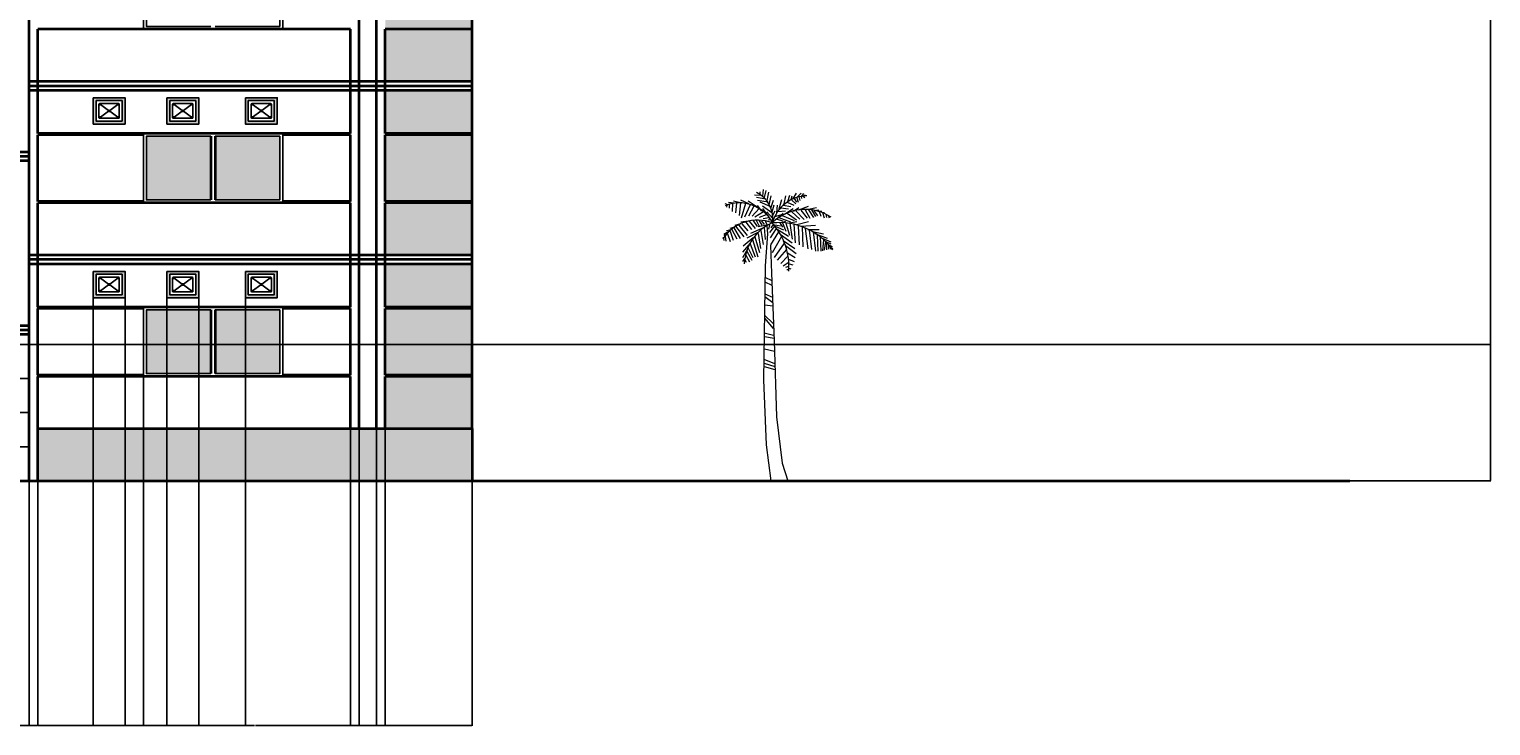
# Model space of a CAD drawing. Units: inches. Extents: x -742 to 1386, y -64 to 951.
# Tile 7 of 8: x 376 to 1386, y -64 to 418. Entities that reach past the tile are written whole.
import ezdxf

# ---------------------------------------------------------------- set-up
doc = ezdxf.new("R2010")
doc.units = ezdxf.units.IN
doc.header["$MEASUREMENT"] = 0
for name, color, linetype, lineweight in [('A-ANNO-DIMS', 2, 'Continuous', 18), ('A-DOOR', 31, 'Continuous', 25), ('A-ELEV', 7, 'Continuous', 35), ('A-ELEV-PATT', 252, 'Continuous', 13), ('A-GLAZ', 4, 'Continuous', 25), ('A-WALL-PATT', 8, 'Continuous', 13), ('tree', 3, 'Continuous', 18)]:
    doc.layers.add(name, color=color, linetype=linetype, lineweight=lineweight)
doc.styles.get("Standard").update_dxf_attribs({"font": 'arial.ttf'})
doc.dimstyles.get("Standard").update_dxf_attribs({"dimtxt": 0.18, "dimasz": 0.18, "dimexe": 0.18, "dimexo": 0.0625, "dimgap": 0.09, "dimtad": 0, "dimtih": 1, "dimtoh": 1, "dimdec": 4, "dimzin": 0, "dimdsep": 46, "dimtxsty": 'Standard', "dimcen": 0.09, "dimadec": 0, "dimazin": 0, "dimtfac": 1, "dimtdec": 4, "dimtofl": 0, "dimtmove": 0, "dimatfit": 3, "dimfxl": 1, "dimtolj": 1, "dimtzin": 0, "dimarcsym": 0})

# ---------------------------------------------------------------- blocks, each defined once
blk = doc.blocks.new('*U2')
for p, q in [((-25.283, 191.751), (-29.342, 192.246)), ((-20.064, 191.751), (-25.863, 193.238)), ((-21.031, 191.998), (-21.804, 183.325)), ((-15.232, 191.255), (-20.644, 193.981)), ((-9.433, 189.025), (-15.618, 193.238)), ((-6.727, 197.202), (-11.366, 197.45)), ((-3.441, 194.477), (-10.013, 195.716)), ((-1.894, 192.494), (-9.24, 193.733)), ((-7.5, 199.68), (-7.5, 197.946)), ((-0.541, 189.52), (-7.307, 192.494)), ((-5.567, 196.707), (-4.987, 201.167)), ((-4.407, 195.716), (-3.247, 200.672)), ((-2.474, 193.733), (-1.315, 199.433)), ((-1.121, 190.759), (0.232, 196.955)), ((0.038, 188.281), (1.778, 193.981)), ((5.837, 187.786), (7.577, 194.229)), ((9.317, 191.255), (10.283, 196.955)), ((11.25, 192.494), (15.889, 190.512)), ((11.829, 192.99), (13.182, 197.45)), ((13.956, 194.229), (14.729, 196.955)), ((14.536, 193.981), (17.242, 191.255)), ((15.116, 194.477), (17.822, 198.689)), ((16.082, 194.972), (17.822, 192.494)), ((18.015, 195.716), (20.914, 198.689)), ((18.015, 195.468), (18.981, 192.494)), ((19.368, 196.459), (19.948, 193.733)), ((20.914, 196.459), (21.301, 194.972)), ((21.301, 196.459), (22.847, 198.441)), ((22.074, 196.707), (23.427, 195.716)), ((23.234, 196.707), (23.62, 197.698)), ((-29.729, 190.759), (-31.469, 191.255)), ((-30.309, 190.512), (-30.695, 189.025)), ((-28.763, 190.759), (-28.763, 188.281)), ((-26.443, 191.503), (-26.636, 186.051)), ((-23.737, 191.751), (-24.51, 185.06)), ((-17.551, 191.503), (-20.451, 181.343)), ((-14.265, 190.759), (-18.131, 182.086)), ((-11.753, 189.768), (-15.425, 182.83)), ((-8.08, 188.034), (-12.912, 182.83)), ((-4.987, 185.803), (-10.979, 182.086)), ((-6.147, 186.299), (-9.24, 190.264)), ((-3.247, 183.821), (-8.08, 181.838)), ((-5.76, 190.016), (0.618, 185.308)), ((-5.76, 188.034), (-1.508, 182.582)), ((-2.668, 185.803), (1.198, 181.343)), ((1.005, 185.803), (2.358, 190.759)), ((1.005, 182.582), (2.938, 186.547)), ((2.938, 182.582), (6.61, 183.821)), ((4.098, 185.06), (4.678, 190.512)), ((4.871, 186.051), (10.09, 186.547)), ((4.871, 181.591), (8.544, 184.812)), ((5.644, 181.838), (13.569, 178.865)), ((6.997, 188.529), (12.216, 187.786)), ((7.77, 183.325), (16.082, 179.856)), ((8.544, 190.512), (13.763, 189.52)), ((9.51, 184.317), (15.502, 188.034)), ((11.25, 184.812), (17.628, 180.352)), ((14.536, 185.803), (19.948, 180.847)), ((15.695, 186.299), (19.368, 188.777)), ((17.242, 186.547), (23.041, 180.599)), ((19.368, 187.29), (26.133, 189.768)), ((20.721, 187.042), (25.167, 181.343)), ((23.814, 187.29), (26.907, 181.343)), ((24.78, 187.538), (31.546, 188.777)), ((26.133, 187.29), (29.419, 181.838)), ((28.066, 187.29), (30.966, 182.582)), ((29.806, 186.795), (32.319, 183.078)), ((29.999, 186.795), (33.092, 187.29)), ((32.512, 186.299), (35.218, 186.299)), ((33.479, 186.051), (34.445, 182.83)), ((35.605, 185.556), (37.151, 185.308)), ((35.798, 185.308), (36.958, 181.591)), ((38.118, 184.317), (38.504, 181.838)), ((39.857, 182.83), (40.244, 181.591)), ((-28.956, 172.174), (-32.435, 170.192)), ((-27.409, 173.413), (-30.695, 172.67)), ((-25.09, 175.148), (-28.376, 174.404)), ((-27.989, 172.422), (-26.056, 166.227)), ((-26.829, 173.661), (-23.544, 167.218)), ((-25.476, 174.652), (-21.224, 167.466)), ((-21.031, 177.626), (-24.897, 176.387)), ((-24.317, 175.891), (-18.711, 168.457)), ((-22.191, 176.635), (-16.391, 169.448)), ((-15.618, 179.36), (-20.644, 178.617)), ((-20.064, 177.626), (-15.812, 172.67)), ((-17.358, 178.617), (-13.299, 173.661)), ((-8.466, 171.678), (-16.585, 167.713)), ((-15.038, 179.36), (-10.786, 174.404)), ((-4.214, 175.148), (-14.072, 170.935)), ((-12.332, 180.104), (-9.433, 175.643)), ((-10.206, 180.104), (-8.08, 175.891)), ((-1.701, 176.882), (-8.66, 175.396)), ((-8.273, 180.104), (-6.147, 176.635)), ((-6.92, 172.917), (-5.374, 163.253)), ((-6.34, 179.608), (-4.6, 177.13)), ((-1.315, 181.591), (-5.374, 181.095)), ((-4.6, 174.9), (-4.021, 166.722)), ((-4.021, 179.36), (-2.861, 177.378)), ((-2.668, 176.387), (-2.376, 170.594)), ((-0.348, 180.352), (-1.894, 180.104)), ((-0.928, 176.882), (-1.508, 173.909)), ((2.551, 175.891), (-0.928, 171.431)), ((3.711, 174.404), (-0.541, 167.961)), ((5.257, 171.926), (-0.155, 163.005)), ((1.585, 177.13), (0.038, 174.652)), ((1.585, 177.13), (6.61, 176.139)), ((2.938, 175.891), (8.737, 173.413)), ((4.098, 180.847), (8.35, 179.608)), ((4.291, 173.909), (12.216, 168.953)), ((6.224, 178.121), (8.157, 175.148)), ((7.384, 178.369), (10.476, 179.36)), ((8.157, 178.121), (10.476, 172.422)), ((10.476, 177.874), (12.796, 169.696)), ((11.829, 177.874), (18.015, 179.113)), ((13.182, 177.874), (14.729, 166.97)), ((15.889, 177.13), (16.855, 164.492)), ((18.015, 177.13), (26.133, 179.113)), ((18.981, 175.891), (19.561, 163.005)), ((20.914, 175.891), (30.966, 176.635)), ((21.688, 175.396), (22.074, 161.518)), ((23.814, 174.404), (25.554, 160.279)), ((25.554, 173.661), (33.285, 173.661)), ((26.52, 173.165), (28.066, 159.784)), ((28.839, 172.174), (36.378, 170.687)), ((29.226, 171.926), (30.966, 158.545)), ((-32.628, 167.961), (-33.208, 167.961)), ((-32.628, 167.713), (-32.435, 165.979)), ((-31.082, 169.944), (-32.435, 169.2)), ((-31.662, 168.705), (-31.082, 165.483)), ((-29.922, 170.687), (-27.989, 165.235)), ((-14.265, 164.244), (-19.678, 158.049)), ((-12.139, 167.961), (-19.098, 162.014)), ((-14.265, 163.749), (-10.786, 154.828)), ((-12.719, 166.722), (-9.046, 154.828)), ((-10.979, 168.457), (-7.887, 157.801)), ((-8.853, 170.935), (-7.113, 160.527)), ((7.384, 168.705), (0.812, 157.553)), ((9.317, 164.244), (2.358, 154.332)), ((6.417, 170.439), (14.729, 164.492)), ((8.544, 165.979), (16.662, 160.527)), ((10.09, 162.51), (17.435, 157.058)), ((30.966, 170.687), (38.891, 167.713)), ((32.126, 169.696), (32.512, 158.545)), ((34.058, 168.705), (34.445, 158.545)), ((35.412, 167.713), (41.404, 164.988)), ((36.378, 166.474), (35.605, 158.792)), ((37.731, 165.235), (36.958, 159.288)), ((37.924, 165.235), (41.404, 163.749)), ((38.504, 164.492), (38.504, 159.536)), ((39.664, 163.253), (42.37, 161.766)), ((39.857, 162.757), (39.857, 160.031)), ((40.824, 161.766), (41.21, 160.031)), ((-16.005, 160.031), (-19.484, 154.084)), ((-18.131, 153.589), (-19.484, 151.606)), ((-17.938, 152.597), (-16.972, 151.111)), ((-17.358, 155.819), (-14.845, 151.358)), ((-16.585, 158.545), (-13.106, 152.35)), ((-15.618, 160.775), (-12.332, 154.332)), ((10.863, 159.784), (4.484, 152.35)), ((11.829, 155.075), (6.804, 150.119)), ((11.443, 157.553), (16.855, 154.332)), ((12.216, 153.093), (16.082, 151.606)), ((41.21, 161.518), (42.757, 160.279)), ((12.603, 151.111), (8.544, 148.385)), ((12.216, 148.137), (10.09, 147.393)), ((12.409, 145.659), (11.056, 145.659)), ((12.409, 146.898), (13.763, 146.402)), ((12.603, 149.872), (15.116, 149.128)), ((-4.081, 140.645), (0.753, 138.261)), ((-4.081, 137.547), (0.753, 135.163)), ((-4.081, 129.205), (1.124, 126.821)), ((-4.081, 127.298), (1.31, 123.246)), ((-4.081, 121.578), (1.31, 120.863)), ((-4.453, 112.283), (1.682, 105.133)), ((-4.267, 114.428), (1.682, 108.708)), ((-4.639, 102.273), (1.868, 100.604)), ((-4.453, 99.651), (2.24, 98.459)), ((-4.453, 91.071), (2.426, 89.641)), ((-4.825, 83.921), (2.612, 81.061)), ((-4.639, 81.299), (2.797, 78.916)), ((-4.639, 78.916), (2.797, 76.771))]:
    blk.add_line(p, q)
for points in [[(-2.363, 170.553), (-3.88, 148.505), (-4.988, 69.634), (-3.325, 24.869), (0, 0)], [(-0.116, 162.848), (0.554, 143.532), (2.217, 96.635), (3.88, 44.054), (7.76, 12.079), (11.64, 0)]]:
    blk.add_lwpolyline(points)
for centre, radius, start, end in [((-21.738, 166.094), 25.899, 27.67115, 112.5305), ((-18.427, 181.448), 19.715, 350.285, 64.11229), ((25.595, 171.567), 25.395, 91.40319, 163.882), ((23.687, 155.341), 32.188, 56.19272, 134.3213), ((-9.259, 151.732), 28.386, 68.38311, 147.5322), ((14.394, 148.393), 32.752, 113.7592, 177.4133), ((5.828, 132.718), 45.639, 35.98777, 95.82273), ((-32.8, 147.923), 45.309, 356.1943, 41.37848)]:
    blk.add_arc(centre, radius, start, end)
blk = doc.blocks.new('VENT-WIN')
h = blk.add_hatch(color=256)
h.dxf.hatch_style = 1
h.paths.add_polyline_path([(11.5, 9.1, 1), (10.5, 9.1, 1)])
h.paths.add_polyline_path([(16.9, 13.7, 1), (18, 13.7, 1)])
h.paths.add_polyline_path([(18, 4.5, 1), (16.9, 4.5, 1)])
h.paths.add_polyline_path([(5, 4.5, 1), (4, 4.5, 1)])
h.paths.add_polyline_path([(4, 13.7, 1), (5, 13.7, 1)])
for p, q in [((5, 13.5), (10.6, 9.4)), ((11.4, 9.4), (17, 13.5)), ((5, 4.7), (10.6, 8.8)), ((11.4, 8.8), (17, 4.7))]:
    blk.add_line(p, q)
for points in [[(0, 18.2), (22, 18.2), (22, 0), (0, 0)], [(2, 16.2), (20, 16.2), (20, 2), (2, 2)]]:
    blk.add_lwpolyline(points, close=True)
for points in [[(4, 4.5), (4, 13.7)], [(4.5, 14.2), (17.5, 14.2)], [(18, 13.7), (18, 4.5)], [(17.5, 4), (4.5, 4)]]:
    blk.add_lwpolyline(points)
for centre in [(4.5, 13.7), (17.5, 13.7), (4.5, 4.5), (11, 9.1), (17.5, 4.5)]:
    blk.add_circle(centre, 0.519)
blk = doc.blocks.new('WIN-1000-2PANE')
blk.add_lwpolyline([(0, 48), (96.2, 48), (96.2, 0), (0, 0)], close=True)
for points in [[(46.6, 2), (2, 2), (2, 46), (46.6, 46)], [(49.6, 46), (94.2, 46), (94.2, 2), (49.6, 2)]]:
    blk.add_lwpolyline(points)
blk = doc.blocks.new('*D15')
at = {"layer": 'A-ANNO-DIMS', "color": 0, "lineweight": -2, "transparency": 16777216}
for p, q in [((262.2, 105.7), (262.2, -63.6)), ((382.2, 105.7), (382.2, -63.6)), ((262.4, -63.4), (321.9, -63.4)), ((382, -63.4), (322.5, -63.4))]:
    blk.add_line(p, q, dxfattribs=at)
at = {"layer": 'A-ANNO-DIMS', "color": 0, "transparency": 16777216}
for points in [[(262.4, -63.4), (262.4, -63.4), (262.2, -63.4)], [(382, -63.4), (382, -63.4), (382.2, -63.4)]]:
    blk.add_solid(points, dxfattribs=at)
at = {"layer": 'Defpoints', "color": 0, "transparency": 16777216}
for p in [(262.2, 105.7), (382.2, 105.7), (382.2, -63.4)]:
    blk.add_point(p, dxfattribs=at)
at = {"layer": 'A-ANNO-DIMS', "color": 0, "transparency": 16777216, "insert": (322.2, -63.4), "char_height": 0.18, "attachment_point": 5}
blk.add_mtext('\\A1;120', dxfattribs=at)
blk = doc.blocks.new('*D16')
at = {"layer": 'A-ANNO-DIMS', "color": 0, "lineweight": -2, "transparency": 16777216}
for p, q in [((382.2, 105.7), (382.2, -63.6)), ((682.2, 105.7), (682.2, -63.6)), ((382.4, -63.4), (531.9, -63.4)), ((682, -63.4), (532.5, -63.4))]:
    blk.add_line(p, q, dxfattribs=at)
at = {"layer": 'A-ANNO-DIMS', "color": 0, "transparency": 16777216}
for points in [[(382.4, -63.4), (382.4, -63.4), (382.2, -63.4)], [(682, -63.4), (682, -63.4), (682.2, -63.4)]]:
    blk.add_solid(points, dxfattribs=at)
at = {"layer": 'Defpoints', "color": 0, "transparency": 16777216}
for p in [(382.2, 105.7), (682.2, 105.7), (682.2, -63.4)]:
    blk.add_point(p, dxfattribs=at)
at = {"layer": 'A-ANNO-DIMS', "color": 0, "transparency": 16777216, "insert": (532.2, -63.4), "char_height": 0.18, "attachment_point": 5}
blk.add_mtext('\\A1;300', dxfattribs=at)
blk = doc.blocks.new('*D21')
at = {"layer": 'A-ANNO-DIMS', "color": 0, "lineweight": -2, "transparency": 16777216}
for p, q in [((598.2, 141.7), (598.2, -63.6)), ((604.2, 141.7), (604.2, -63.6)), ((598.4, -63.4), (601.1, -63.4)), ((604, -63.4), (601.4, -63.4))]:
    blk.add_line(p, q, dxfattribs=at)
at = {"layer": 'A-ANNO-DIMS', "color": 0, "transparency": 16777216}
for points in [[(598.4, -63.4), (598.4, -63.4), (598.2, -63.4)], [(604, -63.4), (604, -63.4), (604.2, -63.4)]]:
    blk.add_solid(points, dxfattribs=at)
at = {"layer": 'Defpoints', "color": 0, "transparency": 16777216}
for p in [(598.2, 141.7), (604.2, 141.7), (604.2, -63.4)]:
    blk.add_point(p, dxfattribs=at)
at = {"layer": 'A-ANNO-DIMS', "color": 0, "transparency": 16777216, "insert": (601.2, -63.4), "char_height": 0.18, "attachment_point": 5}
blk.add_mtext('\\A1;6', dxfattribs=at)
blk = doc.blocks.new('*D22')
at = {"layer": 'A-ANNO-DIMS', "color": 0, "lineweight": -2, "transparency": 16777216}
for p, q in [((604.2, 141.7), (604.2, -63.6)), ((616.2, 141.7), (616.2, -63.6)), ((604.4, -63.4), (610, -63.4)), ((616, -63.4), (610.4, -63.4))]:
    blk.add_line(p, q, dxfattribs=at)
at = {"layer": 'A-ANNO-DIMS', "color": 0, "transparency": 16777216}
for points in [[(604.4, -63.4), (604.4, -63.4), (604.2, -63.4)], [(616, -63.4), (616, -63.4), (616.2, -63.4)]]:
    blk.add_solid(points, dxfattribs=at)
at = {"layer": 'Defpoints', "color": 0, "transparency": 16777216}
for p in [(604.2, 141.7), (616.2, 141.7), (616.2, -63.4)]:
    blk.add_point(p, dxfattribs=at)
at = {"layer": 'A-ANNO-DIMS', "color": 0, "transparency": 16777216, "insert": (610.2, -63.4), "char_height": 0.18, "attachment_point": 5}
blk.add_mtext('\\A1;12', dxfattribs=at)
blk = doc.blocks.new('*D23')
at = {"layer": 'A-ANNO-DIMS', "color": 0, "lineweight": -2, "transparency": 16777216}
for p, q in [((616.2, 141.7), (616.2, -63.6)), ((622.2, 141.7), (622.2, -63.6)), ((616.4, -63.4), (619.1, -63.4)), ((622, -63.4), (619.4, -63.4))]:
    blk.add_line(p, q, dxfattribs=at)
at = {"layer": 'A-ANNO-DIMS', "color": 0, "transparency": 16777216}
for points in [[(616.4, -63.4), (616.4, -63.4), (616.2, -63.4)], [(622, -63.4), (622, -63.4), (622.2, -63.4)]]:
    blk.add_solid(points, dxfattribs=at)
at = {"layer": 'Defpoints', "color": 0, "transparency": 16777216}
for p in [(616.2, 141.7), (622.2, 141.7), (622.2, -63.4)]:
    blk.add_point(p, dxfattribs=at)
at = {"layer": 'A-ANNO-DIMS', "color": 0, "transparency": 16777216, "insert": (619.2, -63.4), "char_height": 0.18, "attachment_point": 5}
blk.add_mtext('\\A1;6', dxfattribs=at)
blk = doc.blocks.new('*D24')
at = {"layer": 'A-ANNO-DIMS', "color": 0, "lineweight": -2, "transparency": 16777216}
for p, q in [((622.2, 141.7), (622.2, -63.6)), ((682.2, 141.7), (682.2, -63.6)), ((622.4, -63.4), (652, -63.4)), ((682, -63.4), (652.4, -63.4))]:
    blk.add_line(p, q, dxfattribs=at)
at = {"layer": 'A-ANNO-DIMS', "color": 0, "transparency": 16777216}
for points in [[(622.4, -63.4), (622.4, -63.4), (622.2, -63.4)], [(682, -63.4), (682, -63.4), (682.2, -63.4)]]:
    blk.add_solid(points, dxfattribs=at)
at = {"layer": 'Defpoints', "color": 0, "transparency": 16777216}
for p in [(622.2, 141.7), (682.2, 141.7), (682.2, -63.4)]:
    blk.add_point(p, dxfattribs=at)
at = {"layer": 'A-ANNO-DIMS', "color": 0, "transparency": 16777216, "insert": (652.2, -63.4), "char_height": 0.18, "attachment_point": 5}
blk.add_mtext('\\A1;60', dxfattribs=at)
blk = doc.blocks.new('*D29')
at = {"layer": 'A-ANNO-DIMS', "color": 0, "lineweight": -2, "transparency": 16777216}
for p, q in [((382.2, 178.7), (382.2, -63.6)), ((455.1, 178.7), (455.1, -63.6)), ((382.4, -63.4), (418.3, -63.4)), ((455, -63.4), (419.1, -63.4))]:
    blk.add_line(p, q, dxfattribs=at)
at = {"layer": 'A-ANNO-DIMS', "color": 0, "transparency": 16777216}
for points in [[(382.4, -63.4), (382.4, -63.4), (382.2, -63.4)], [(455, -63.4), (455, -63.4), (455.1, -63.4)]]:
    blk.add_solid(points, dxfattribs=at)
at = {"layer": 'Defpoints', "color": 0, "transparency": 16777216}
for p in [(382.2, 178.7), (455.1, 178.7), (455.1, -63.4)]:
    blk.add_point(p, dxfattribs=at)
at = {"layer": 'A-ANNO-DIMS', "color": 0, "transparency": 16777216, "insert": (418.7, -63.4), "char_height": 0.18, "attachment_point": 5}
blk.add_mtext('\\A1;72.91', dxfattribs=at)
blk = doc.blocks.new('*D30')
at = {"layer": 'A-ANNO-DIMS', "color": 0, "lineweight": -2, "transparency": 16777216}
for p, q in [((382.2, 225.7), (382.2, -63.6)), ((420.4, 232.2), (420.4, -63.6)), ((382.4, -63.4), (401, -63.4)), ((420.2, -63.4), (401.6, -63.4))]:
    blk.add_line(p, q, dxfattribs=at)
at = {"layer": 'A-ANNO-DIMS', "color": 0, "transparency": 16777216}
for points in [[(382.4, -63.4), (382.4, -63.4), (382.2, -63.4)], [(420.2, -63.4), (420.2, -63.4), (420.4, -63.4)]]:
    blk.add_solid(points, dxfattribs=at)
at = {"layer": 'Defpoints', "color": 0, "transparency": 16777216}
for p in [(382.2, 225.7), (420.4, 232.2), (420.4, -63.4)]:
    blk.add_point(p, dxfattribs=at)
at = {"layer": 'A-ANNO-DIMS', "color": 0, "transparency": 16777216, "insert": (401.3, -63.4), "char_height": 0.18, "attachment_point": 5}
blk.add_mtext('\\A1;38.2', dxfattribs=at)
blk = doc.blocks.new('*D31')
at = {"layer": 'A-ANNO-DIMS', "color": 0, "lineweight": -2, "transparency": 16777216}
for p, q in [((442.4, 232.2), (442.4, -63.6)), ((471.3, 232.2), (471.3, -63.6)), ((442.6, -63.4), (456.5, -63.4)), ((471.1, -63.4), (457.2, -63.4))]:
    blk.add_line(p, q, dxfattribs=at)
at = {"layer": 'A-ANNO-DIMS', "color": 0, "transparency": 16777216}
for points in [[(442.6, -63.4), (442.6, -63.4), (442.4, -63.4)], [(471.1, -63.4), (471.1, -63.4), (471.3, -63.4)]]:
    blk.add_solid(points, dxfattribs=at)
at = {"layer": 'Defpoints', "color": 0, "transparency": 16777216}
for p in [(442.4, 232.2), (471.3, 232.2), (471.3, -63.4)]:
    blk.add_point(p, dxfattribs=at)
at = {"layer": 'A-ANNO-DIMS', "color": 0, "transparency": 16777216, "insert": (456.9, -63.4), "char_height": 0.18, "attachment_point": 5}
blk.add_mtext('\\A1;28.91', dxfattribs=at)
blk = doc.blocks.new('*D32')
at = {"layer": 'A-ANNO-DIMS', "color": 0, "lineweight": -2, "transparency": 16777216}
for p, q in [((493.3, 232.2), (493.3, -63.6)), ((525.6, 232.2), (525.6, -63.6)), ((493.5, -63.4), (509, -63.4)), ((525.4, -63.4), (509.9, -63.4))]:
    blk.add_line(p, q, dxfattribs=at)
at = {"layer": 'A-ANNO-DIMS', "color": 0, "transparency": 16777216}
for points in [[(493.5, -63.4), (493.5, -63.4), (493.3, -63.4)], [(525.4, -63.4), (525.4, -63.4), (525.6, -63.4)]]:
    blk.add_solid(points, dxfattribs=at)
at = {"layer": 'Defpoints', "color": 0, "transparency": 16777216}
for p in [(493.3, 232.2), (525.6, 232.2), (525.6, -63.4)]:
    blk.add_point(p, dxfattribs=at)
at = {"layer": 'A-ANNO-DIMS', "color": 0, "transparency": 16777216, "insert": (509.4, -63.4), "char_height": 0.18, "attachment_point": 5}
blk.add_mtext('\\A1;32.263', dxfattribs=at)
blk = doc.blocks.new('*D35')
at = {"layer": 'A-ANNO-DIMS', "color": 0, "lineweight": -2, "transparency": 16777216}
for p, q in [((343.2, 199.8), (343.2, -63.6)), ((376.2, 199.8), (376.2, -63.6)), ((343.4, -63.4), (359.3, -63.4)), ((376, -63.4), (360.2, -63.4))]:
    blk.add_line(p, q, dxfattribs=at)
at = {"layer": 'A-ANNO-DIMS', "color": 0, "transparency": 16777216}
for points in [[(343.4, -63.4), (343.4, -63.4), (343.2, -63.4)], [(376, -63.4), (376, -63.4), (376.2, -63.4)]]:
    blk.add_solid(points, dxfattribs=at)
at = {"layer": 'Defpoints', "color": 0, "transparency": 16777216}
for p in [(343.2, 199.8), (376.2, 199.8), (376.2, -63.4)]:
    blk.add_point(p, dxfattribs=at)
at = {"layer": 'A-ANNO-DIMS', "color": 0, "transparency": 16777216, "insert": (359.7, -63.4), "char_height": 0.18, "attachment_point": 5}
blk.add_mtext('\\A1;32.985', dxfattribs=at)
blk = doc.blocks.new('*D39')
at = {"layer": 'A-ANNO-DIMS', "color": 0, "lineweight": -2, "transparency": 16777216}
for p, q in [((391.3, 853.8), (1386, 853.8)), ((1385.8, 853.6), (1385.8, 479.9)), ((1385.8, 105.9), (1385.8, 479.6)), ((682.3, 105.7), (1386, 105.7))]:
    blk.add_line(p, q, dxfattribs=at)
at = {"layer": 'A-ANNO-DIMS', "color": 0, "transparency": 16777216}
for points in [[(1385.8, 853.6), (1385.9, 853.6), (1385.8, 853.8)], [(1385.8, 105.9), (1385.9, 105.9), (1385.8, 105.7)]]:
    blk.add_solid(points, dxfattribs=at)
at = {"layer": 'Defpoints', "color": 0, "transparency": 16777216}
for p in [(391.2, 853.8), (682.2, 105.7), (1385.8, 105.7)]:
    blk.add_point(p, dxfattribs=at)
at = {"layer": 'A-ANNO-DIMS', "color": 0, "transparency": 16777216, "insert": (1385.8, 479.8), "char_height": 0.18, "attachment_point": 5}
blk.add_mtext('\\A1;748', dxfattribs=at)
blk = doc.blocks.new('*D51')
at = {"layer": 'A-ANNO-DIMS', "color": 0, "lineweight": -2, "transparency": 16777216}
for p, q in [((376.3, 199.8), (1386, 199.8)), ((1385.8, 199.7), (1385.8, 153)), ((1385.8, 105.9), (1385.8, 152.6)), ((376.3, 105.7), (1386, 105.7))]:
    blk.add_line(p, q, dxfattribs=at)
at = {"layer": 'A-ANNO-DIMS', "color": 0, "transparency": 16777216}
for points in [[(1385.8, 199.7), (1385.9, 199.7), (1385.8, 199.8)], [(1385.8, 105.9), (1385.9, 105.9), (1385.8, 105.7)]]:
    blk.add_solid(points, dxfattribs=at)
at = {"layer": 'Defpoints', "color": 0, "transparency": 16777216}
for p in [(376.2, 199.8), (376.2, 105.7), (1385.8, 105.7)]:
    blk.add_point(p, dxfattribs=at)
at = {"layer": 'A-ANNO-DIMS', "color": 0, "transparency": 16777216, "insert": (1385.8, 152.8), "char_height": 0.18, "attachment_point": 5}
blk.add_mtext('\\A1;94.1', dxfattribs=at)

msp = doc.modelspace()

# ---------------------------------------------------------------- hatches: boundary and pattern name
at = {"layer": 'A-ELEV-PATT'}
h = msp.add_hatch(color=256, dxfattribs=at)
h.dxf.hatch_style = 1
h.paths.add_polyline_path([(442.4136, 370.4496), (420.4263, 370.4496), (420.4263, 352.2254), (442.4136, 352.2254)])
h.paths.add_polyline_path([(440.4136, 354.2254), (422.4263, 354.2254), (422.4263, 368.4496), (440.4136, 368.4496)], flags=16)
h.paths.add_polyline_path([(493.3109, 370.4496), (471.3236, 370.4496), (471.3236, 352.2254), (493.3109, 352.2254)])
h.paths.add_polyline_path([(491.3109, 368.4496), (491.3109, 354.2254), (473.3236, 354.2254), (473.3236, 368.4496)], flags=16)
h.paths.add_polyline_path([(547.5617, 370.4496), (525.5743, 370.4496), (525.5743, 352.2254), (547.5617, 352.2254)])
h.paths.add_polyline_path([(545.5617, 368.4496), (545.5617, 354.2254), (527.5743, 354.2254), (527.5743, 368.4496)], flags=16)
h = msp.add_hatch(color=256, dxfattribs=at)
h.dxf.hatch_style = 1
h.set_gradient(color1=(0, 255, 255), name='CURVED')
h.paths.add_polyline_path([(139.7128, 343.7399), (95.1117, 343.7399), (95.1117, 299.7399), (139.7128, 299.7399)])
h.paths.add_polyline_path([(187.3139, 343.7399), (142.7128, 343.7399), (142.7128, 299.7399), (187.3139, 299.7399)])
h.paths.add_polyline_path([(501.7423, 343.7399), (457.1413, 343.7399), (457.1413, 299.7399), (501.7423, 299.7399)])
h.paths.add_polyline_path([(549.3434, 343.7399), (504.7423, 343.7399), (504.7423, 299.7399), (549.3434, 299.7399)])
h = msp.add_hatch(color=256, dxfattribs=at)
h.dxf.hatch_style = 1
h.paths.add_polyline_path([(442.4136, 250.4496), (420.4263, 250.4496), (420.4263, 232.2254), (442.4136, 232.2254)])
h.paths.add_polyline_path([(440.4136, 234.2254), (422.4263, 234.2254), (422.4263, 248.4496), (440.4136, 248.4496)], flags=16)
h.paths.add_polyline_path([(493.3109, 250.4496), (471.3236, 250.4496), (471.3236, 232.2254), (493.3109, 232.2254)])
h.paths.add_polyline_path([(491.3109, 248.4496), (491.3109, 234.2254), (473.3236, 234.2254), (473.3236, 248.4496)], flags=16)
h.paths.add_polyline_path([(547.5617, 250.4496), (525.5743, 250.4496), (525.5743, 232.2254), (547.5617, 232.2254)])
h.paths.add_polyline_path([(545.5617, 248.4496), (545.5617, 234.2254), (527.5743, 234.2254), (527.5743, 248.4496)], flags=16)
h = msp.add_hatch(color=256, dxfattribs=at)
h.dxf.hatch_style = 1
h.set_gradient(color1=(0, 255, 255), tint=1, name='CURVED')
h.paths.add_polyline_path([(139.7128, 223.7399), (95.1117, 223.7399), (95.1117, 179.7399), (139.7128, 179.7399)])
h.paths.add_polyline_path([(187.3139, 223.7399), (142.7128, 223.7399), (142.7128, 179.7399), (187.3139, 179.7399)])
h.paths.add_polyline_path([(501.7423, 223.7399), (457.1413, 223.7399), (457.1413, 179.7399), (501.7423, 179.7399)])
h.paths.add_polyline_path([(549.3434, 223.7399), (504.7423, 223.7399), (504.7423, 179.7399), (549.3434, 179.7399)])
at = {"layer": 'A-WALL-PATT', "transparency": 33554457}
h = msp.add_hatch(dxfattribs=at)
h.set_pattern_fill('AR-B88', color=256)
h.paths.add_polyline_path([(22.2276, 224.7399), (-37.7724, 224.7399), (-37.7724, 178.7399), (22.2276, 178.7399)])
h.paths.add_polyline_path([(22.2276, 177.7399), (-37.7724, 177.7399), (-37.7724, 141.7399), (22.2276, 141.7399)])
h.paths.add_polyline_path([(22.2276, 255.7399), (-37.7724, 255.7399), (-37.7724, 225.7399), (22.2276, 225.7399)])
h.paths.add_polyline_path([(22.2276, 297.7399), (-37.7724, 297.7399), (-37.7724, 261.7399), (22.2276, 261.7399)])
h.paths.add_polyline_path([(22.2276, 344.7399), (-37.7724, 344.7399), (-37.7724, 298.7399), (22.2276, 298.7399)])
h.paths.add_polyline_path([(22.2276, 375.7399), (-37.7724, 375.7399), (-37.7724, 345.7399), (22.2276, 345.7399)])
h.paths.add_polyline_path([(22.2276, 417.7399), (-37.7724, 417.7399), (-37.7724, 381.7399), (22.2276, 381.7399)])
h.paths.add_polyline_path([(22.2276, 464.7399), (-37.7724, 464.7399), (-37.7724, 418.7399), (22.2276, 418.7399)])
h.paths.add_polyline_path([(22.2276, 495.7399), (-37.7724, 495.7399), (-37.7724, 465.7399), (22.2276, 465.7399)])
h.paths.add_polyline_path([(22.2276, 537.7399), (-37.7724, 537.7399), (-37.7724, 501.7399), (22.2276, 501.7399)])
h.paths.add_polyline_path([(22.2276, 584.7399), (-37.7724, 584.7399), (-37.7724, 538.7399), (22.2276, 538.7399)])
h.paths.add_polyline_path([(22.2276, 615.7399), (-37.7724, 615.7399), (-37.7724, 585.7399), (22.2276, 585.7399)])
h.paths.add_polyline_path([(22.2276, 657.7399), (-37.7724, 657.7399), (-37.7724, 621.7399), (22.2276, 621.7399)])
h.paths.add_polyline_path([(22.2276, 704.7399), (-37.7724, 704.7399), (-37.7724, 658.7399), (22.2276, 658.7399)])
h.paths.add_polyline_path([(22.2276, 735.7399), (-37.7724, 735.7399), (-37.7724, 705.7399), (22.2276, 705.7399)])
h.paths.add_polyline_path([(376.2276, 835.7799), (268.2276, 835.7799), (268.2276, 806.8548), (376.2276, 806.8548)])
h.paths.add_polyline_path([(682.2276, 735.7399), (622.2276, 735.7399), (622.2276, 705.7399), (682.2276, 705.7399)])
h.paths.add_polyline_path([(682.2276, 704.7399), (622.2276, 704.7399), (622.2276, 658.7399), (682.2276, 658.7399)])
h.paths.add_polyline_path([(682.2276, 657.7399), (622.2276, 657.7399), (622.2276, 621.7399), (682.2276, 621.7399)])
h.paths.add_polyline_path([(682.2276, 615.7399), (622.2276, 615.7399), (622.2276, 585.7399), (682.2276, 585.7399)])
h.paths.add_polyline_path([(682.2276, 584.7399), (622.2276, 584.7399), (622.2276, 538.7399), (682.2276, 538.7399)])
h.paths.add_polyline_path([(682.2276, 537.7399), (622.2276, 537.7399), (622.2276, 501.7399), (682.2276, 501.7399)])
h.paths.add_polyline_path([(682.2276, 495.7399), (622.2276, 495.7399), (622.2276, 465.7399), (682.2276, 465.7399)])
h.paths.add_polyline_path([(682.2276, 464.7399), (622.2276, 464.7399), (622.2276, 418.7399), (682.2276, 418.7399)])
h.paths.add_polyline_path([(682.2276, 417.7399), (622.2276, 417.7399), (622.2276, 381.7399), (682.2276, 381.7399)])
h.paths.add_polyline_path([(682.2276, 375.7399), (622.2276, 375.7399), (622.2276, 345.7399), (682.2276, 345.7399)])
h.paths.add_polyline_path([(682.2276, 344.7399), (622.2276, 344.7399), (622.2276, 298.7399), (682.2276, 298.7399)])
h.paths.add_polyline_path([(682.2276, 297.7399), (622.2276, 297.7399), (622.2276, 261.7399), (682.2276, 261.7399)])
h.paths.add_polyline_path([(682.2276, 255.7399), (622.2276, 255.7399), (622.2276, 225.7399), (682.2276, 225.7399)])
h.paths.add_polyline_path([(682.2276, 224.7399), (622.2276, 224.7399), (622.2276, 178.7399), (682.2276, 178.7399)])
h.paths.add_polyline_path([(682.2276, 177.7399), (622.2276, 177.7399), (622.2276, 141.7399), (682.2276, 141.7399)])
h = msp.add_hatch(dxfattribs=at)
h.set_pattern_fill('GRAVEL', color=256, scale=40)
h.paths.add_polyline_path([(262.2276, 141.7399), (-37.7724, 141.7399), (-37.7724, 105.7399), (262.2276, 105.7399)])
h.paths.add_polyline_path([(682.2276, 141.7399), (382.2276, 141.7399), (382.2276, 105.7399), (682.2276, 105.7399)])

# ---------------------------------------------------------------- linework, layer by layer
at = {"layer": 'A-DOOR'}
for p, q in [((343.2429, 199.8339), (376.2276, 199.8339)), ((343.2429, 176.3104), (376.2276, 176.3104)), ((343.2429, 152.7869), (376.2276, 152.7869)), ((343.2429, 129.2634), (376.2276, 129.2634)), ((268.2276, 105.7399), (376.2276, 105.7399))]:
    msp.add_line(p, q, dxfattribs=at)
at = {"layer": 'A-ELEV'}
for p, q in [((376.2276, 105.7399), (376.2276, 835.7799)), ((604.2276, 141.7399), (604.2276, 741.7399)), ((616.2276, 141.7399), (616.2276, 741.7399)), ((682.2276, 141.7399), (682.2276, 741.7399)), ((598.2276, 417.7399), (382.2276, 417.7399)), ((382.2276, 345.7399), (382.2276, 417.7399)), ((598.2276, 345.7399), (598.2276, 417.7399)), ((682.2276, 417.7399), (622.2276, 417.7399)), ((622.2276, 345.7399), (622.2276, 417.7399)), ((376.2276, 381.7399), (682.2276, 381.7399)), ((376.2276, 378.7399), (682.2276, 378.7399)), ((376.2276, 375.7399), (682.2276, 375.7399)), ((598.2276, 345.7399), (382.2276, 345.7399)), ((455.1413, 344.7399), (382.2276, 344.7399)), ((382.2276, 298.7399), (382.2276, 344.7399)), ((501.7423, 343.7399), (501.7423, 299.7399)), ((504.7423, 343.7399), (504.7423, 299.7399)), ((598.2276, 344.7399), (551.3434, 344.7399)), ((598.2276, 298.7399), (598.2276, 344.7399)), ((682.2276, 345.7399), (622.2276, 345.7399)), ((682.2276, 344.7399), (622.2276, 344.7399)), ((622.2276, 298.7399), (622.2276, 344.7399)), ((376.2276, 332.8548), (268.2276, 332.8548)), ((376.2276, 329.8548), (268.2276, 329.8548)), ((376.2276, 326.8548), (268.2276, 326.8548)), ((455.1413, 298.7399), (382.2276, 298.7399)), ((382.2276, 225.7399), (382.2276, 297.7399)), ((598.2276, 297.7399), (382.2276, 297.7399)), ((598.2276, 298.7399), (551.3434, 298.7399)), ((598.2276, 255.7399), (598.2276, 297.7399)), ((682.2276, 298.7399), (622.2276, 298.7399)), ((682.2276, 297.7399), (622.2276, 297.7399)), ((622.2276, 255.7399), (622.2276, 297.7399)), ((376.2276, 261.7399), (622.2276, 261.7399)), ((376.2276, 258.7399), (622.2276, 258.7399)), ((376.2276, 255.7399), (622.2276, 255.7399)), ((598.2276, 225.7399), (598.2276, 255.7399)), ((622.2276, 261.7399), (682.2276, 261.7399)), ((622.2276, 258.7399), (682.2276, 258.7399)), ((622.2276, 225.7399), (622.2276, 255.7399)), ((622.2276, 255.7399), (682.2276, 255.7399)), ((598.2276, 225.7399), (382.2276, 225.7399)), ((455.1413, 224.7399), (382.2276, 224.7399)), ((382.2276, 178.7399), (382.2276, 224.7399)), ((501.7423, 223.7399), (501.7423, 179.7399)), ((504.7423, 223.7399), (504.7423, 179.7399)), ((598.2276, 224.7399), (551.3434, 224.7399)), ((598.2276, 178.7399), (598.2276, 224.7399)), ((682.2276, 225.7399), (622.2276, 225.7399)), ((682.2276, 224.7399), (622.2276, 224.7399)), ((622.2276, 178.7399), (622.2276, 224.7399)), ((376.2276, 212.8548), (268.2276, 212.8548)), ((376.2276, 209.8548), (268.2276, 209.8548)), ((376.2276, 206.8548), (268.2276, 206.8548)), ((455.1413, 178.7399), (382.2276, 178.7399)), ((382.2276, 105.7399), (382.2276, 177.7399)), ((598.2276, 177.7399), (382.2276, 177.7399)), ((598.2276, 178.7399), (551.3434, 178.7399)), ((598.2276, 141.7399), (598.2276, 177.7399)), ((682.2276, 178.7399), (622.2276, 178.7399)), ((622.2276, 141.7399), (622.2276, 177.7399)), ((682.2276, 177.7399), (622.2276, 177.7399)), ((382.2276, 141.7399), (682.2276, 141.7399)), ((682.2276, 141.7399), (682.2276, 105.7399)), ((262.2276, 105.7399), (682.2276, 105.7399)), ((682.2276, 105.7399), (1288.5762, 105.7399))]:
    msp.add_line(p, q, dxfattribs=at)

# ---------------------------------------------------------------- block references
at = {"layer": 'A-GLAZ', "extrusion": (0, 0, -1), "zscale": -1}
for p in [(-551.3432, 417.74), (-551.3432, 297.74), (-551.3432, 177.74)]:
    msp.add_blockref('WIN-1000-2PANE', p, dxfattribs=at)
at = {"layer": 'A-GLAZ'}
for p in [(420.4267, 352.225), (471.324, 352.225), (525.5748, 352.225), (420.4267, 232.225), (471.324, 232.225), (525.5748, 232.225)]:
    msp.add_blockref('VENT-WIN', p, dxfattribs=at)
at = {"layer": 'tree'}
msp.add_blockref('*U2', (888.6275, 105.7399), dxfattribs=at)

# ---------------------------------------------------------------- dimensions: what is measured, and where the dimension line sits
at = {"layer": 'A-ANNO-DIMS'}
for p1, p2, override, picture, middle in [((391.2276, 853.7799), (682.2276, 105.7399), {"dimdec": 0, "dimlfac": 1, "dimrnd": 0, "dimzin": 0, "dimdsep": 46, "dimlunit": 2}, '*D39', (1385.8262, 479.7599)), ((376.2276, 199.8339), (376.2276, 105.7399), {"dimdec": 1, "dimlfac": 1, "dimrnd": 0, "dimzin": 0, "dimdsep": 46, "dimlunit": 2}, '*D51', (1385.8262, 152.7869))]:
    dim = msp.add_linear_dim(base=(1385.8262, 105.7399), p1=p1, p2=p2, angle=90, dimstyle='Standard', override=override, dxfattribs=at)
    dim.commit()
    dim.dimension.update_dxf_attribs({"geometry": picture, "text_midpoint": middle})
for base, p1, p2, override, picture, middle in [((420.4263, -63.3971), (382.2276, 225.7399), (420.4263, 232.2254), {"dimdec": 1, "dimlfac": 1, "dimrnd": 0, "dimzin": 0, "dimdsep": 46, "dimlunit": 2}, '*D30', (401.3269, -63.3971)), ((471.3236, -63.3971), (442.4136, 232.2254), (471.3236, 232.2254), {"dimdec": 2, "dimlfac": 1, "dimrnd": 0, "dimzin": 0, "dimdsep": 46, "dimlunit": 2}, '*D31', (456.8686, -63.3971)), ((525.5743, -63.3971), (493.3109, 232.2254), (525.5743, 232.2254), {"dimdec": 3, "dimlfac": 1, "dimrnd": 0, "dimzin": 0, "dimdsep": 46, "dimlunit": 2}, '*D32', (509.4426, -63.3971)), ((376.2276, -63.3971), (343.2429, 199.8339), (376.2276, 199.8339), {"dimdec": 3, "dimlfac": 1, "dimrnd": 0, "dimzin": 0, "dimdsep": 46, "dimlunit": 2}, '*D35', (359.7352, -63.3971)), ((455.1413, -63.3971), (382.2276, 178.7399), (455.1413, 178.7399), {"dimdec": 2, "dimlfac": 1, "dimrnd": 0, "dimzin": 0, "dimdsep": 46, "dimlunit": 2}, '*D29', (418.6844, -63.3971)), ((604.2276, -63.3971), (598.2276, 141.7399), (604.2276, 141.7399), {"dimdec": 0, "dimlfac": 1, "dimrnd": 0, "dimzin": 0, "dimdsep": 46, "dimlunit": 2}, '*D21', (601.2276, -63.3971)), ((616.2276, -63.3971), (604.2276, 141.7399), (616.2276, 141.7399), {"dimdec": 0, "dimlfac": 1, "dimrnd": 0, "dimzin": 0, "dimdsep": 46, "dimlunit": 2}, '*D22', (610.2276, -63.3971)), ((622.2276, -63.3971), (616.2276, 141.7399), (622.2276, 141.7399), {"dimdec": 0, "dimlfac": 1, "dimrnd": 0, "dimzin": 0, "dimdsep": 46, "dimlunit": 2}, '*D23', (619.2276, -63.3971)), ((682.2276, -63.3971), (622.2276, 141.7399), (682.2276, 141.7399), {"dimdec": 0, "dimlfac": 1, "dimrnd": 0, "dimzin": 0, "dimdsep": 46, "dimlunit": 2}, '*D24', (652.2276, -63.3971)), ((382.2276, -63.3971), (262.2276, 105.7399), (382.2276, 105.7399), {"dimdec": 0, "dimlfac": 1, "dimrnd": 0, "dimzin": 0, "dimdsep": 46, "dimlunit": 2}, '*D15', (322.2276, -63.3971)), ((682.2276, -63.3971), (382.2276, 105.7399), (682.2276, 105.7399), {"dimdec": 0, "dimlfac": 1, "dimrnd": 0, "dimzin": 0, "dimdsep": 46, "dimlunit": 2}, '*D16', (532.2276, -63.3971))]:
    dim = msp.add_linear_dim(base=base, p1=p1, p2=p2, dimstyle='Standard', override=override, dxfattribs=at)
    dim.commit()
    dim.dimension.update_dxf_attribs({"geometry": picture, "text_midpoint": middle})

doc.saveas('drawing.dxf')
